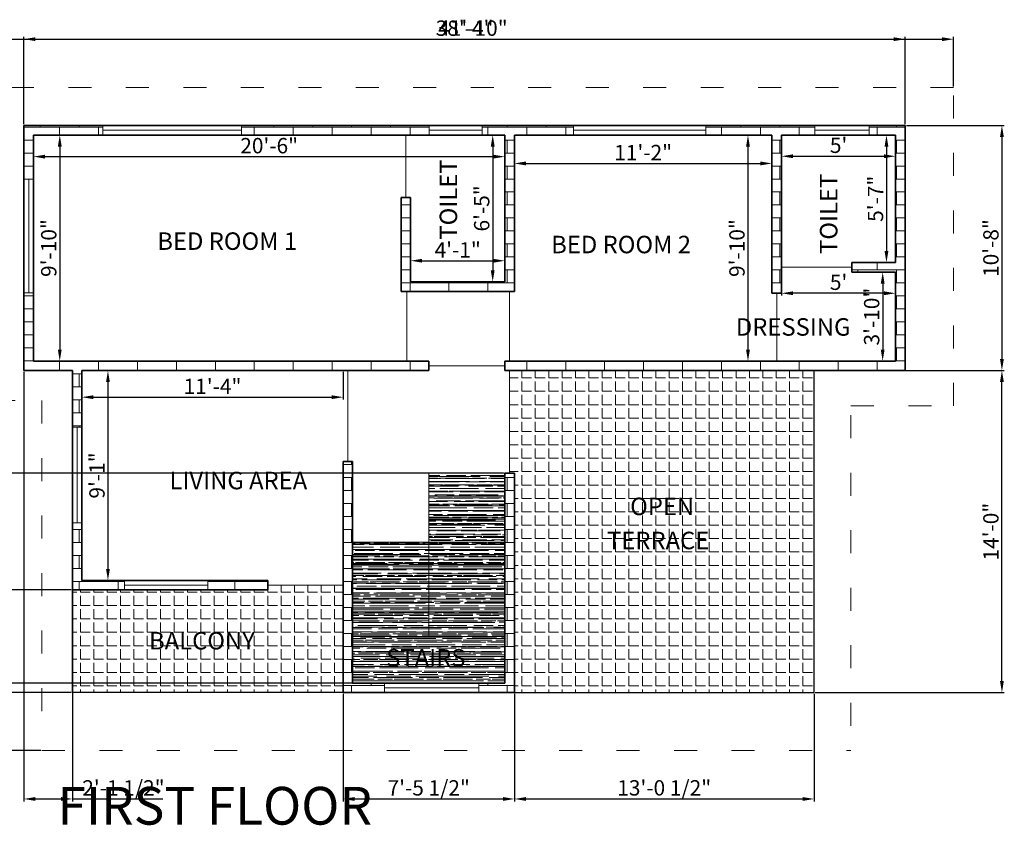
# Model space of a CAD drawing. Units: millimetres. Extents: x 1518 to 2850, y 936 to 2174.
# Tile 5 of 5: x 2336 to 2850, y 1715 to 2136. Entities that reach past the tile are written whole.
import ezdxf

# ---------------------------------------------------------------- set-up
doc = ezdxf.new("R2010")
doc.units = ezdxf.units.MM
doc.linetypes.add('ACAD_ISO03W100', pattern=[30, 12, -18])
for name, color, linetype, lineweight, true_color in [('A-ANNO-DIMS', 9, 'Continuous', 18, 0xafd9aa), ('A-ANNO-TEXT', 85, 'Continuous', 25, 0x58ba48), ('A-AREA-IDEN', 31, 'Continuous', 18, 0xfecc66), ('A-DOOR', 244, 'Continuous', 20, 0x991b1e), ('A-FLOR-PATT', 252, 'Continuous', 13, 0x939598), ('A-GLAZ', 141, 'Continuous', 18, 0xadddf7), ('A-ROOF-OVHD', 177, 'ACAD_ISO03W100', 18, 0x293189)]:
    doc.layers.add(name, color=color, linetype=linetype, lineweight=lineweight, true_color=true_color)
for name, color, linetype, lineweight in [('A-FLOR', 7, 'Continuous', 25), ('A-FLOR-STRS', 7, 'Continuous', 20), ('A-FLOR-STRS-PATT', 7, 'Continuous', 13), ('A-WALL', 7, 'Continuous', 35), ('A-WALL-PATT', 7, 'Continuous', 13)]:
    doc.layers.add(name, color=color, linetype=linetype, lineweight=lineweight)
doc.styles.get("Standard").update_dxf_attribs({"font": 'arial.ttf'})
doc.dimstyles.new('ISO-25', dxfattribs={"dimtxt": 8, "dimasz": 6, "dimexe": 1.25, "dimexo": 0.625, "dimtad": 1, "dimdec": 0, "dimlunit": 3, "dimtxsty": 'Standard', "dimcen": 2.5, "dimadec": 0, "dimazin": 0, "dimtfac": 1, "dimtdec": 0, "dimtmove": 0, "dimatfit": 3, "dimfxl": 1, "dimarcsym": 0})

# ---------------------------------------------------------------- blocks, each defined once
blk = doc.blocks.new('*D14')
at = {"layer": 'A-ANNO-DIMS', "color": 0, "lineweight": -2, "transparency": 16777216}
for p, q in [((2343.49, 2074.9), (2343.49, 2062.99)), ((2589.49, 2074.9), (2589.49, 2062.99)), ((2349.49, 2064.24), (2583.49, 2064.24))]:
    blk.add_line(p, q, dxfattribs=at)
at = {"layer": 'A-ANNO-DIMS', "color": 0, "transparency": 16777216}
for points in [[(2349.49, 2065.24), (2349.49, 2063.24), (2343.49, 2064.24)], [(2583.49, 2065.24), (2583.49, 2063.24), (2589.49, 2064.24)]]:
    blk.add_solid(points, dxfattribs=at)
at = {"layer": 'Defpoints', "color": 0, "transparency": 16777216}
for p in [(2343.49, 2075.52), (2589.49, 2075.52), (2589.49, 2064.24)]:
    blk.add_point(p, dxfattribs=at)
at = {"layer": 'A-ANNO-DIMS', "color": 0, "transparency": 16777216, "insert": (2466.49, 2068.95), "char_height": 8, "attachment_point": 5}
blk.add_mtext('20\'-6"', dxfattribs=at)
blk = doc.blocks.new('*D15')
at = {"layer": 'A-ANNO-DIMS', "color": 0, "lineweight": -2, "transparency": 16777216}
for p, q in [((2344.11, 2075.52), (2358.43, 2075.52)), ((2357.18, 2069.52), (2357.18, 1963.6)), ((2344.11, 1957.6), (2358.43, 1957.6))]:
    blk.add_line(p, q, dxfattribs=at)
at = {"layer": 'A-ANNO-DIMS', "color": 0, "transparency": 16777216}
for points in [[(2356.18, 2069.52), (2358.18, 2069.52), (2357.18, 2075.52)], [(2356.18, 1963.6), (2358.18, 1963.6), (2357.18, 1957.6)]]:
    blk.add_solid(points, dxfattribs=at)
at = {"layer": 'Defpoints', "color": 0, "transparency": 16777216}
for p in [(2343.49, 2075.52), (2343.49, 1957.6), (2357.18, 1957.6)]:
    blk.add_point(p, dxfattribs=at)
at = {"layer": 'A-ANNO-DIMS', "color": 0, "transparency": 16777216, "insert": (2352.47, 2016.56), "char_height": 8, "attachment_point": 5, "rotation": 90}
blk.add_mtext('9\'-10"', dxfattribs=at)
blk = doc.blocks.new('*D16')
at = {"layer": 'A-ANNO-DIMS', "color": 0, "lineweight": -2, "transparency": 16777216}
for p, q in [((2588.86, 2075.52), (2581.93, 2075.52)), ((2583.18, 2069.52), (2583.18, 2004.95)), ((2588.86, 1998.95), (2581.93, 1998.95))]:
    blk.add_line(p, q, dxfattribs=at)
at = {"layer": 'A-ANNO-DIMS', "color": 0, "transparency": 16777216}
for points in [[(2582.18, 2069.52), (2584.18, 2069.52), (2583.18, 2075.52)], [(2582.18, 2004.95), (2584.18, 2004.95), (2583.18, 1998.95)]]:
    blk.add_solid(points, dxfattribs=at)
at = {"layer": 'Defpoints', "color": 0, "transparency": 16777216}
for p in [(2589.49, 2075.52), (2583.18, 1998.95), (2589.49, 1998.95)]:
    blk.add_point(p, dxfattribs=at)
at = {"layer": 'A-ANNO-DIMS', "color": 0, "transparency": 16777216, "insert": (2578.47, 2037.24), "char_height": 8, "attachment_point": 5, "rotation": 90}
blk.add_mtext('6\'-5"', dxfattribs=at)
blk = doc.blocks.new('*D17')
at = {"layer": 'A-ANNO-DIMS', "color": 0, "lineweight": -2, "transparency": 16777216}
for p, q in [((2540.33, 1999.58), (2540.33, 2011.19)), ((2546.33, 2009.94), (2583.49, 2009.94)), ((2589.49, 1999.58), (2589.49, 2011.19))]:
    blk.add_line(p, q, dxfattribs=at)
at = {"layer": 'A-ANNO-DIMS', "color": 0, "transparency": 16777216}
for points in [[(2546.33, 2010.94), (2546.33, 2008.94), (2540.33, 2009.94)], [(2583.49, 2010.94), (2583.49, 2008.94), (2589.49, 2009.94)]]:
    blk.add_solid(points, dxfattribs=at)
at = {"layer": 'Defpoints', "color": 0, "transparency": 16777216}
for p in [(2589.49, 2009.94), (2540.33, 1998.95), (2589.49, 1998.95)]:
    blk.add_point(p, dxfattribs=at)
at = {"layer": 'A-ANNO-DIMS', "color": 0, "transparency": 16777216, "insert": (2564.91, 2014.59), "char_height": 8, "attachment_point": 5}
blk.add_mtext('4\'-1"', dxfattribs=at)
blk = doc.blocks.new('*D18')
at = {"layer": 'A-ANNO-DIMS', "color": 0, "lineweight": -2, "transparency": 16777216}
for p, q in [((2594.49, 2074.9), (2594.49, 2059.46)), ((2728.96, 2074.9), (2728.96, 2059.46)), ((2600.49, 2060.71), (2722.96, 2060.71))]:
    blk.add_line(p, q, dxfattribs=at)
at = {"layer": 'A-ANNO-DIMS', "color": 0, "transparency": 16777216}
for points in [[(2600.49, 2061.71), (2600.49, 2059.71), (2594.49, 2060.71)], [(2722.96, 2061.71), (2722.96, 2059.71), (2728.96, 2060.71)]]:
    blk.add_solid(points, dxfattribs=at)
at = {"layer": 'Defpoints', "color": 0, "transparency": 16777216}
for p in [(2594.49, 2075.52), (2728.96, 2075.52), (2728.96, 2060.71)]:
    blk.add_point(p, dxfattribs=at)
at = {"layer": 'A-ANNO-DIMS', "color": 0, "transparency": 16777216, "insert": (2661.72, 2065.35), "char_height": 8, "attachment_point": 5}
blk.add_mtext('11\'-2"', dxfattribs=at)
blk = doc.blocks.new('*D19')
at = {"layer": 'A-ANNO-DIMS', "color": 0, "lineweight": -2, "transparency": 16777216}
for p, q in [((2728.33, 2075.52), (2715.17, 2075.52)), ((2716.42, 2069.52), (2716.42, 1963.6)), ((2728.33, 1957.6), (2715.17, 1957.6))]:
    blk.add_line(p, q, dxfattribs=at)
at = {"layer": 'A-ANNO-DIMS', "color": 0, "transparency": 16777216}
for points in [[(2715.42, 2069.52), (2717.42, 2069.52), (2716.42, 2075.52)], [(2715.42, 1963.6), (2717.42, 1963.6), (2716.42, 1957.6)]]:
    blk.add_solid(points, dxfattribs=at)
at = {"layer": 'Defpoints', "color": 0, "transparency": 16777216}
for p in [(2728.96, 2075.52), (2716.42, 1957.6), (2728.96, 1957.6)]:
    blk.add_point(p, dxfattribs=at)
at = {"layer": 'A-ANNO-DIMS', "color": 0, "transparency": 16777216, "insert": (2711.71, 2016.56), "char_height": 8, "attachment_point": 5, "rotation": 90}
blk.add_mtext('9\'-10"', dxfattribs=at)
blk = doc.blocks.new('*D20')
at = {"layer": 'A-ANNO-DIMS', "color": 0, "lineweight": -2, "transparency": 16777216}
for p, q in [((2733.96, 2074.9), (2733.96, 2063.2)), ((2793.49, 2074.9), (2793.49, 2063.2)), ((2739.96, 2064.45), (2787.49, 2064.45))]:
    blk.add_line(p, q, dxfattribs=at)
at = {"layer": 'A-ANNO-DIMS', "color": 0, "transparency": 16777216}
for points in [[(2739.96, 2065.45), (2739.96, 2063.45), (2733.96, 2064.45)], [(2787.49, 2065.45), (2787.49, 2063.45), (2793.49, 2064.45)]]:
    blk.add_solid(points, dxfattribs=at)
at = {"layer": 'Defpoints', "color": 0, "transparency": 16777216}
for p in [(2733.96, 2075.52), (2793.49, 2075.52), (2793.49, 2064.45)]:
    blk.add_point(p, dxfattribs=at)
at = {"layer": 'A-ANNO-DIMS', "color": 0, "transparency": 16777216, "insert": (2763.72, 2069.15), "char_height": 8, "attachment_point": 5}
blk.add_mtext("5'", dxfattribs=at)
blk = doc.blocks.new('*D21')
at = {"layer": 'A-ANNO-DIMS', "color": 0, "lineweight": -2, "transparency": 16777216}
for p, q in [((2792.86, 2075.52), (2787.47, 2075.52)), ((2788.72, 2069.52), (2788.72, 2015.01)), ((2792.86, 2009.01), (2787.47, 2009.01))]:
    blk.add_line(p, q, dxfattribs=at)
at = {"layer": 'A-ANNO-DIMS', "color": 0, "transparency": 16777216}
for points in [[(2787.72, 2069.52), (2789.72, 2069.52), (2788.72, 2075.52)], [(2787.72, 2015.01), (2789.72, 2015.01), (2788.72, 2009.01)]]:
    blk.add_solid(points, dxfattribs=at)
at = {"layer": 'Defpoints', "color": 0, "transparency": 16777216}
for p in [(2793.49, 2075.52), (2788.72, 2009.01), (2793.49, 2009.01)]:
    blk.add_point(p, dxfattribs=at)
at = {"layer": 'A-ANNO-DIMS', "color": 0, "transparency": 16777216, "insert": (2784.03, 2042.27), "char_height": 8, "attachment_point": 5, "rotation": 90}
blk.add_mtext('5\'-7"', dxfattribs=at)
blk = doc.blocks.new('*D22')
at = {"layer": 'A-ANNO-DIMS', "color": 0, "lineweight": -2, "transparency": 16777216}
for p, q in [((2733.96, 2003.39), (2733.96, 1991.73)), ((2793.49, 2003.39), (2793.49, 1991.73)), ((2787.49, 1992.98), (2739.96, 1992.98))]:
    blk.add_line(p, q, dxfattribs=at)
at = {"layer": 'A-ANNO-DIMS', "color": 0, "transparency": 16777216}
for points in [[(2739.96, 1993.98), (2739.96, 1991.98), (2733.96, 1992.98)], [(2787.49, 1993.98), (2787.49, 1991.98), (2793.49, 1992.98)]]:
    blk.add_solid(points, dxfattribs=at)
at = {"layer": 'Defpoints', "color": 0, "transparency": 16777216}
for p in [(2733.96, 2004.01), (2793.49, 2004.01), (2733.96, 1992.98)]:
    blk.add_point(p, dxfattribs=at)
at = {"layer": 'A-ANNO-DIMS', "color": 0, "transparency": 16777216, "insert": (2763.72, 1997.67), "char_height": 8, "attachment_point": 5}
blk.add_mtext("5'", dxfattribs=at)
blk = doc.blocks.new('*D23')
at = {"layer": 'A-ANNO-DIMS', "color": 0, "lineweight": -2, "transparency": 16777216}
for p, q in [((2792.86, 2004.01), (2785.49, 2004.01)), ((2786.74, 1998.01), (2786.74, 1963.6)), ((2792.86, 1957.6), (2785.49, 1957.6))]:
    blk.add_line(p, q, dxfattribs=at)
at = {"layer": 'A-ANNO-DIMS', "color": 0, "transparency": 16777216}
for points in [[(2785.74, 1998.01), (2787.74, 1998.01), (2786.74, 2004.01)], [(2785.74, 1963.6), (2787.74, 1963.6), (2786.74, 1957.6)]]:
    blk.add_solid(points, dxfattribs=at)
at = {"layer": 'Defpoints', "color": 0, "transparency": 16777216}
for p in [(2793.49, 2004.01), (2786.74, 1957.6), (2793.49, 1957.6)]:
    blk.add_point(p, dxfattribs=at)
at = {"layer": 'A-ANNO-DIMS', "color": 0, "transparency": 16777216, "insert": (2782.03, 1980.8), "char_height": 8, "attachment_point": 5, "rotation": 90}
blk.add_mtext('3\'-10"', dxfattribs=at)
blk = doc.blocks.new('*D24')
at = {"layer": 'A-ANNO-DIMS', "color": 0, "lineweight": -2, "transparency": 16777216}
for p, q in [((2369.38, 1952.6), (2383.59, 1952.6)), ((2382.34, 1946.6), (2382.34, 1849.2)), ((2369.38, 1843.2), (2383.59, 1843.2))]:
    blk.add_line(p, q, dxfattribs=at)
at = {"layer": 'A-ANNO-DIMS', "color": 0, "transparency": 16777216}
for points in [[(2381.34, 1946.6), (2383.34, 1946.6), (2382.34, 1952.6)], [(2381.34, 1849.2), (2383.34, 1849.2), (2382.34, 1843.2)]]:
    blk.add_solid(points, dxfattribs=at)
at = {"layer": 'Defpoints', "color": 0, "transparency": 16777216}
for p in [(2368.76, 1952.6), (2368.76, 1843.2), (2382.34, 1843.2)]:
    blk.add_point(p, dxfattribs=at)
at = {"layer": 'A-ANNO-DIMS', "color": 0, "transparency": 16777216, "insert": (2377.63, 1897.9), "char_height": 8, "attachment_point": 5, "rotation": 90}
blk.add_mtext('9\'-1"', dxfattribs=at)
blk = doc.blocks.new('*D25')
at = {"layer": 'A-ANNO-DIMS', "color": 0, "lineweight": -2, "transparency": 16777216}
for p, q in [((2368.76, 1951.97), (2368.76, 1937.5)), ((2505.07, 1951.97), (2505.07, 1937.5)), ((2374.76, 1938.75), (2499.07, 1938.75))]:
    blk.add_line(p, q, dxfattribs=at)
at = {"layer": 'A-ANNO-DIMS', "color": 0, "transparency": 16777216}
for points in [[(2374.76, 1939.75), (2374.76, 1937.75), (2368.76, 1938.75)], [(2499.07, 1939.75), (2499.07, 1937.75), (2505.07, 1938.75)]]:
    blk.add_solid(points, dxfattribs=at)
at = {"layer": 'Defpoints', "color": 0, "transparency": 16777216}
for p in [(2368.76, 1952.6), (2505.07, 1952.6), (2505.07, 1938.75)]:
    blk.add_point(p, dxfattribs=at)
at = {"layer": 'A-ANNO-DIMS', "color": 0, "transparency": 16777216, "insert": (2436.92, 1943.39), "char_height": 8, "attachment_point": 5}
blk.add_mtext('11\'-4"', dxfattribs=at)
blk = doc.blocks.new('*D42')
at = {"layer": 'A-ANNO-DIMS', "color": 0, "lineweight": -2, "transparency": 16777216}
for p, q in [((2338.49, 2081.15), (2338.49, 2126.78)), ((2344.49, 2125.53), (2792.49, 2125.53)), ((2798.49, 2081.15), (2798.49, 2126.78))]:
    blk.add_line(p, q, dxfattribs=at)
at = {"layer": 'A-ANNO-DIMS', "color": 0, "transparency": 16777216}
for points in [[(2344.49, 2126.53), (2344.49, 2124.53), (2338.49, 2125.53)], [(2792.49, 2126.53), (2792.49, 2124.53), (2798.49, 2125.53)]]:
    blk.add_solid(points, dxfattribs=at)
at = {"layer": 'Defpoints', "color": 0, "transparency": 16777216}
for p in [(2798.49, 2125.53), (2338.49, 2080.52), (2798.49, 2080.52)]:
    blk.add_point(p, dxfattribs=at)
at = {"layer": 'A-ANNO-DIMS', "color": 0, "transparency": 16777216, "insert": (2568.49, 2130.24), "char_height": 8, "attachment_point": 5}
blk.add_mtext('38\'-4"', dxfattribs=at)
blk = doc.blocks.new('*D43')
at = {"layer": 'A-ANNO-DIMS', "color": 0, "lineweight": -2, "transparency": 16777216}
for p, q in [((2799.11, 2080.52), (2850.23, 2080.52)), ((2848.98, 2074.52), (2848.98, 1958.6)), ((2799.11, 1952.6), (2850.23, 1952.6))]:
    blk.add_line(p, q, dxfattribs=at)
at = {"layer": 'A-ANNO-DIMS', "color": 0, "transparency": 16777216}
for points in [[(2847.98, 2074.52), (2849.98, 2074.52), (2848.98, 2080.52)], [(2847.98, 1958.6), (2849.98, 1958.6), (2848.98, 1952.6)]]:
    blk.add_solid(points, dxfattribs=at)
at = {"layer": 'Defpoints', "color": 0, "transparency": 16777216}
for p in [(2798.49, 2080.52), (2798.49, 1952.6), (2848.98, 1952.6)]:
    blk.add_point(p, dxfattribs=at)
at = {"layer": 'A-ANNO-DIMS', "color": 0, "transparency": 16777216, "insert": (2844.27, 2016.56), "char_height": 8, "attachment_point": 5, "rotation": 90}
blk.add_mtext('10\'-8"', dxfattribs=at)
blk = doc.blocks.new('*D44')
at = {"layer": 'A-ANNO-DIMS', "color": 0, "lineweight": -2, "transparency": 16777216}
for p, q in [((2338.49, 1951.97), (2338.49, 1727.89)), ((2363.76, 1951.97), (2363.76, 1727.89)), ((2344.49, 1729.14), (2357.76, 1729.14)), ((2363.76, 1729.14), (2411.05, 1729.14))]:
    blk.add_line(p, q, dxfattribs=at)
at = {"layer": 'A-ANNO-DIMS', "color": 0, "transparency": 16777216}
for points in [[(2344.49, 1730.14), (2344.49, 1728.14), (2338.49, 1729.14)], [(2357.76, 1730.14), (2357.76, 1728.14), (2363.76, 1729.14)]]:
    blk.add_solid(points, dxfattribs=at)
at = {"layer": 'Defpoints', "color": 0, "transparency": 16777216}
for p in [(2338.49, 1952.6), (2363.76, 1952.6), (2363.76, 1729.14)]:
    blk.add_point(p, dxfattribs=at)
at = {"layer": 'A-ANNO-DIMS', "color": 0, "transparency": 16777216, "insert": (2390.41, 1733.9), "char_height": 8, "attachment_point": 5}
blk.add_mtext('2\'-1 1/2"', dxfattribs=at)
blk = doc.blocks.new('*D45')
at = {"layer": 'A-ANNO-DIMS', "color": 0, "lineweight": -2, "transparency": 16777216}
for p, q in [((2505.07, 1783.97), (2505.07, 1727.89)), ((2594.49, 1783.97), (2594.49, 1727.89)), ((2511.07, 1729.14), (2588.49, 1729.14))]:
    blk.add_line(p, q, dxfattribs=at)
at = {"layer": 'A-ANNO-DIMS', "color": 0, "transparency": 16777216}
for points in [[(2511.07, 1730.14), (2511.07, 1728.14), (2505.07, 1729.14)], [(2588.49, 1730.14), (2588.49, 1728.14), (2594.49, 1729.14)]]:
    blk.add_solid(points, dxfattribs=at)
at = {"layer": 'Defpoints', "color": 0, "transparency": 16777216}
for p in [(2505.07, 1784.6), (2594.49, 1784.6), (2594.49, 1729.14)]:
    blk.add_point(p, dxfattribs=at)
at = {"layer": 'A-ANNO-DIMS', "color": 0, "transparency": 16777216, "insert": (2549.78, 1733.9), "char_height": 8, "attachment_point": 5}
blk.add_mtext('7\'-5 1/2"', dxfattribs=at)
blk = doc.blocks.new('*D46')
at = {"layer": 'A-ANNO-DIMS', "color": 0, "lineweight": -2, "transparency": 16777216}
for p, q in [((2594.49, 1783.97), (2594.49, 1727.89)), ((2750.92, 1783.97), (2750.92, 1727.89)), ((2600.49, 1729.14), (2744.92, 1729.14))]:
    blk.add_line(p, q, dxfattribs=at)
at = {"layer": 'A-ANNO-DIMS', "color": 0, "transparency": 16777216}
for points in [[(2600.49, 1730.14), (2600.49, 1728.14), (2594.49, 1729.14)], [(2744.92, 1730.14), (2744.92, 1728.14), (2750.92, 1729.14)]]:
    blk.add_solid(points, dxfattribs=at)
at = {"layer": 'Defpoints', "color": 0, "transparency": 16777216}
for p in [(2594.49, 1784.6), (2750.92, 1784.6), (2750.92, 1729.14)]:
    blk.add_point(p, dxfattribs=at)
at = {"layer": 'A-ANNO-DIMS', "color": 0, "transparency": 16777216, "insert": (2672.7, 1733.91), "char_height": 8, "attachment_point": 5}
blk.add_mtext('13\'-0 1/2"', dxfattribs=at)
blk = doc.blocks.new('*D47')
at = {"layer": 'A-ANNO-DIMS', "color": 0, "lineweight": -2, "transparency": 16777216}
for p, q in [((2751.54, 1952.6), (2850.23, 1952.6)), ((2848.98, 1790.6), (2848.98, 1946.6)), ((2751.54, 1784.6), (2850.23, 1784.6))]:
    blk.add_line(p, q, dxfattribs=at)
at = {"layer": 'A-ANNO-DIMS', "color": 0, "transparency": 16777216}
for points in [[(2847.98, 1946.6), (2849.98, 1946.6), (2848.98, 1952.6)], [(2847.98, 1790.6), (2849.98, 1790.6), (2848.98, 1784.6)]]:
    blk.add_solid(points, dxfattribs=at)
at = {"layer": 'Defpoints', "color": 0, "transparency": 16777216}
for p in [(2750.92, 1952.6), (2848.98, 1952.6), (2750.92, 1784.6)]:
    blk.add_point(p, dxfattribs=at)
at = {"layer": 'A-ANNO-DIMS', "color": 0, "transparency": 16777216, "insert": (2844.27, 1868.6), "char_height": 8, "attachment_point": 5, "rotation": 90}
blk.add_mtext('14\'-0"', dxfattribs=at)
blk = doc.blocks.new('*D48')
at = {"layer": 'A-ANNO-DIMS', "color": 0, "lineweight": -2, "transparency": 16777216}
for p, q in [((2588.86, 1899.05), (2295.47, 1899.05)), ((2296.72, 1795.6), (2296.72, 1893.05)), ((2588.86, 1789.6), (2295.47, 1789.6))]:
    blk.add_line(p, q, dxfattribs=at)
at = {"layer": 'A-ANNO-DIMS', "color": 0, "transparency": 16777216}
for points in [[(2295.72, 1893.05), (2297.72, 1893.05), (2296.72, 1899.05)], [(2295.72, 1795.6), (2297.72, 1795.6), (2296.72, 1789.6)]]:
    blk.add_solid(points, dxfattribs=at)
at = {"layer": 'Defpoints', "color": 0, "transparency": 16777216}
for p in [(2296.72, 1899.05), (2589.49, 1899.05), (2589.49, 1789.6)]:
    blk.add_point(p, dxfattribs=at)
at = {"layer": 'A-ANNO-DIMS', "color": 0, "transparency": 16777216, "insert": (2291.96, 1844.32), "char_height": 8, "attachment_point": 5, "rotation": 90}
blk.add_mtext('9\'-1 1/2"', dxfattribs=at)
blk = doc.blocks.new('*D49')
at = {"layer": 'A-ANNO-DIMS', "color": 0, "lineweight": -2, "transparency": 16777216}
for p, q in [((2363.13, 1838.2), (2295.47, 1838.2)), ((2296.72, 1790.6), (2296.72, 1832.2)), ((2363.13, 1784.6), (2295.47, 1784.6))]:
    blk.add_line(p, q, dxfattribs=at)
at = {"layer": 'A-ANNO-DIMS', "color": 0, "transparency": 16777216}
for points in [[(2295.72, 1832.2), (2297.72, 1832.2), (2296.72, 1838.2)], [(2295.72, 1790.6), (2297.72, 1790.6), (2296.72, 1784.6)]]:
    blk.add_solid(points, dxfattribs=at)
at = {"layer": 'Defpoints', "color": 0, "transparency": 16777216}
for p in [(2296.72, 1838.2), (2363.76, 1838.2), (2363.76, 1784.6)]:
    blk.add_point(p, dxfattribs=at)
at = {"layer": 'A-ANNO-DIMS', "color": 0, "transparency": 16777216, "insert": (2291.96, 1811.4), "char_height": 8, "attachment_point": 5, "rotation": 90}
blk.add_mtext('4\'-5 1/2"', dxfattribs=at)
blk = doc.blocks.new('*D50')
at = {"layer": 'A-ANNO-DIMS', "color": 0, "lineweight": -2, "transparency": 16777216}
for p, q in [((2321.97, 2100.9), (2321.97, 2126.78)), ((2327.97, 2125.53), (2817.73, 2125.53)), ((2823.73, 2100.9), (2823.73, 2126.78))]:
    blk.add_line(p, q, dxfattribs=at)
at = {"layer": 'A-ANNO-DIMS', "color": 0, "transparency": 16777216}
for points in [[(2327.97, 2126.53), (2327.97, 2124.53), (2321.97, 2125.53)], [(2817.73, 2126.53), (2817.73, 2124.53), (2823.73, 2125.53)]]:
    blk.add_solid(points, dxfattribs=at)
at = {"layer": 'Defpoints', "color": 0, "transparency": 16777216}
for p in [(2823.73, 2125.53), (2321.97, 2100.28), (2823.73, 2100.28)]:
    blk.add_point(p, dxfattribs=at)
at = {"layer": 'A-ANNO-DIMS', "color": 0, "transparency": 16777216, "insert": (2572.85, 2130.24), "char_height": 8, "attachment_point": 5}
blk.add_mtext('41\'-10"', dxfattribs=at)
blk = doc.blocks.new('*D51')
at = {"layer": 'A-ANNO-DIMS', "color": 0, "lineweight": -2, "transparency": 16777216}
for p, q in [((2321.34, 2100.28), (2295.47, 2100.28)), ((2296.72, 2094.28), (2296.72, 1760.39)), ((2347.23, 1754.39), (2295.47, 1754.39))]:
    blk.add_line(p, q, dxfattribs=at)
at = {"layer": 'A-ANNO-DIMS', "color": 0, "transparency": 16777216}
for points in [[(2295.72, 2094.28), (2297.72, 2094.28), (2296.72, 2100.28)], [(2295.72, 1760.39), (2297.72, 1760.39), (2296.72, 1754.39)]]:
    blk.add_solid(points, dxfattribs=at)
at = {"layer": 'Defpoints', "color": 0, "transparency": 16777216}
for p in [(2321.97, 2100.28), (2296.72, 1754.39), (2347.86, 1754.39)]:
    blk.add_point(p, dxfattribs=at)
at = {"layer": 'A-ANNO-DIMS', "color": 0, "transparency": 16777216, "insert": (2292.01, 1927.34), "char_height": 8, "attachment_point": 5, "rotation": 90}
blk.add_mtext('28\'-10"', dxfattribs=at)

msp = doc.modelspace()

# ---------------------------------------------------------------- hatches: boundary and pattern name
at = {"layer": 'A-FLOR-PATT'}
h = msp.add_hatch(dxfattribs=at)
h.set_pattern_fill('ANGLE', color=256)
h.set_pattern_definition([(0, (0, 0), (0, 6.985), [5.08, -1.905]), (90, (0, 0), (-6.985, 4e-16), [5.08, -1.905])])
h.paths.add_polyline_path([(2505.07, 1838.2), (2505.07, 1840.7), (2465.77, 1840.7), (2465.77, 1838.2), (2363.76, 1838.2), (2363.76, 1784.6), (2505.07, 1784.6)])
h.paths.add_polyline_path([(2750.92, 1952.6), (2594.49, 1952.6), (2591.99, 1952.6), (2591.99, 1899.05), (2594.49, 1899.05), (2594.49, 1784.6), (2750.92, 1784.6)])
at = {"layer": 'A-FLOR-STRS-PATT'}
h = msp.add_hatch(dxfattribs=at)
h.set_pattern_fill('AR-RROOF', color=256, scale=0.1)
h.paths.add_polyline_path([(2549.78, 1863.05), (2510.07, 1863.05), (2510.07, 1851.05), (2549.78, 1851.05)])
h.paths.add_polyline_path([(2589.49, 1899.05), (2549.78, 1899.05), (2549.78, 1887.05), (2589.49, 1887.05)])
h.paths.add_polyline_path([(2589.49, 1887.05), (2549.78, 1887.05), (2549.78, 1875.05), (2589.49, 1875.05)])
h.paths.add_polyline_path([(2589.49, 1875.05), (2549.78, 1875.05), (2549.78, 1863.05), (2589.49, 1863.05)])
h.paths.add_polyline_path([(2589.49, 1863.05), (2549.78, 1863.05), (2549.78, 1851.05), (2589.49, 1851.05)])
h.paths.add_polyline_path([(2589.49, 1851.05), (2549.78, 1851.05), (2549.78, 1839.05), (2589.49, 1839.05)])
h.paths.add_polyline_path([(2589.49, 1839.05), (2549.78, 1839.05), (2549.78, 1827.05), (2589.49, 1827.05)])
h.paths.add_polyline_path([(2589.49, 1827.05), (2549.78, 1827.05), (2549.78, 1813.9), (2589.49, 1813.9)])
h.paths.add_polyline_path([(2589.49, 1813.9), (2549.78, 1813.9), (2510.07, 1813.9), (2510.07, 1789.6), (2589.49, 1789.6)])
h.paths.add_polyline_path([(2549.78, 1827.05), (2510.07, 1827.05), (2510.07, 1813.9), (2549.78, 1813.9)])
h.paths.add_polyline_path([(2549.78, 1839.05), (2510.07, 1839.05), (2510.07, 1827.05), (2549.78, 1827.05)])
h.paths.add_polyline_path([(2549.78, 1851.05), (2510.07, 1851.05), (2510.07, 1839.05), (2549.78, 1839.05)])
at = {"layer": 'A-WALL-PATT'}
h = msp.add_hatch(dxfattribs=at)
h.set_pattern_fill('AR-BRSTD', color=256, scale=0.1)
h.paths.add_polyline_path([(2550.01, 2080.52), (2452.04, 2080.52), (2452.04, 2075.52), (2535.33, 2075.52), (2540.33, 2075.52), (2550.01, 2075.52)])
h.paths.add_polyline_path([(2379.7, 2080.52), (2338.49, 2080.52), (2338.49, 2052.54), (2343.49, 2052.54), (2343.49, 2075.52), (2379.7, 2075.52)])
h.paths.add_polyline_path([(2549.78, 1957.6), (2343.49, 1957.6), (2343.49, 1993.2), (2338.49, 1993.2), (2338.49, 1952.6), (2363.76, 1952.6), (2363.76, 1923.14), (2368.76, 1923.14), (2368.76, 1952.6), (2505.07, 1952.6), (2510.07, 1952.6), (2549.78, 1952.6)])
h.paths.add_polyline_path([(2625.42, 2080.52), (2594.49, 2080.52), (2577.67, 2080.52), (2577.67, 2075.52), (2589.49, 2075.52), (2589.49, 1998.95), (2540.33, 1998.95), (2540.33, 2043), (2535.33, 2043), (2535.33, 1993.95), (2589.49, 1993.95), (2594.49, 1993.92), (2594.49, 2075.52), (2625.42, 2075.52)])
h.paths.add_polyline_path([(2751.28, 2080.52), (2694.39, 2080.52), (2694.39, 2075.52), (2728.96, 2075.52), (2728.96, 1992.98), (2733.96, 1992.98), (2733.96, 2004.01), (2733.96, 2009.01), (2733.96, 2075.52), (2751.28, 2075.52)], flags=17)
h.paths.add_polyline_path([(2798.49, 2080.52), (2779.63, 2080.52), (2779.63, 2075.52), (2793.49, 2075.52), (2793.49, 2009.01), (2770.7, 2009.01), (2770.7, 2004.01), (2793.49, 2004.01), (2793.49, 1957.6), (2733.96, 1957.6), (2728.96, 1957.6), (2594.49, 1957.6), (2589.49, 1957.6), (2589.49, 1952.6), (2594.49, 1952.6), (2798.49, 1952.6)])
h.paths.add_polyline_path([(2368.76, 1873.29), (2363.76, 1873.29), (2363.76, 1838.2), (2391.06, 1838.2), (2391.06, 1843.2), (2368.76, 1843.2)])
h.paths.add_polyline_path([(2465.77, 1843.2), (2434.42, 1843.2), (2434.42, 1838.2), (2465.77, 1838.2)])
h.paths.add_polyline_path([(2510.07, 1905.25), (2505.07, 1905.25), (2505.07, 1843.2), (2505.07, 1838.2), (2505.07, 1784.6), (2526.69, 1784.6), (2526.69, 1789.6), (2510.07, 1789.6), (2510.07, 1838.2), (2510.07, 1839.05)])
h.paths.add_polyline_path([(2594.49, 1899.05), (2589.49, 1899.05), (2589.49, 1887.05), (2589.49, 1789.6), (2575.94, 1789.6), (2575.94, 1784.6), (2594.49, 1784.6)])

# ---------------------------------------------------------------- linework, layer by layer
at = {"layer": 'A-DOOR'}
for p, q in [((2537.83, 2043), (2537.83, 2075.52)), ((2770.7, 2006.51), (2733.96, 2006.51)), ((2538.39, 1993.95), (2538.39, 1957.6)), ((2591.99, 1957.6), (2591.99, 1993.92)), ((2731.46, 1992.98), (2731.46, 1957.6)), ((2549.78, 1955.1), (2589.49, 1955.1)), ((2507.57, 1905.25), (2507.57, 1952.6)), ((2591.99, 1899.05), (2591.99, 1952.6)), ((2465.77, 1840.7), (2505.07, 1840.7))]:
    msp.add_line(p, q, dxfattribs=at)
at = {"layer": 'A-FLOR'}
for p, q in [((2750.92, 1784.6), (2750.92, 1952.6)), ((2363.76, 1784.6), (2363.76, 1838.2)), ((2505.07, 1784.6), (2363.76, 1784.6)), ((2594.49, 1784.6), (2750.92, 1784.6))]:
    msp.add_line(p, q, dxfattribs=at)
at = {"layer": 'A-FLOR-STRS'}
for p, q in [((2549.78, 1813.9), (2549.78, 1899.05)), ((2549.78, 1899.05), (2589.49, 1899.05)), ((2589.49, 1899.05), (2589.49, 1887.05)), ((2589.49, 1887.05), (2549.78, 1887.05)), ((2549.78, 1887.05), (2549.78, 1875.05)), ((2549.78, 1875.05), (2589.49, 1875.05)), ((2589.49, 1875.05), (2589.49, 1863.05)), ((2589.49, 1863.05), (2510.07, 1863.05)), ((2510.07, 1863.05), (2510.07, 1851.05)), ((2510.07, 1851.05), (2589.49, 1851.05)), ((2589.49, 1851.05), (2589.49, 1839.05)), ((2589.49, 1839.05), (2510.07, 1839.05)), ((2510.07, 1839.05), (2510.07, 1827.05)), ((2510.07, 1827.05), (2589.49, 1827.05)), ((2510.07, 1813.9), (2589.49, 1813.9))]:
    msp.add_line(p, q, dxfattribs=at)
at = {"layer": 'A-GLAZ'}
for p, q in [((2379.7, 2078.02), (2452.04, 2078.02)), ((2550.01, 2078.02), (2577.67, 2078.02)), ((2625.42, 2078.02), (2694.39, 2078.02)), ((2751.28, 2078.02), (2779.63, 2078.02)), ((2340.99, 1993.2), (2340.99, 2052.54)), ((2366.26, 1873.29), (2366.26, 1923.14)), ((2391.06, 1840.7), (2434.42, 1840.7)), ((2526.69, 1787.1), (2575.94, 1787.1))]:
    msp.add_line(p, q, dxfattribs=at)
for points in [[(2379.7, 2080.52), (2452.04, 2080.52), (2452.04, 2075.52), (2379.7, 2075.52)], [(2550.01, 2080.52), (2577.67, 2080.52), (2577.67, 2075.52), (2550.01, 2075.52)], [(2625.42, 2080.52), (2694.39, 2080.52), (2694.39, 2075.52), (2625.42, 2075.52)], [(2751.28, 2080.52), (2779.63, 2080.52), (2779.63, 2075.52), (2751.28, 2075.52)], [(2338.49, 2052.54), (2343.49, 2052.54), (2343.49, 1993.2), (2338.49, 1993.2)], [(2363.76, 1923.14), (2368.76, 1923.14), (2368.76, 1873.29), (2363.76, 1873.29)], [(2391.06, 1843.2), (2434.42, 1843.2), (2434.42, 1838.2), (2391.06, 1838.2)], [(2526.69, 1789.6), (2575.94, 1789.6), (2575.94, 1784.6), (2526.69, 1784.6)]]:
    msp.add_lwpolyline(points, close=True, dxfattribs=at)
at = {"layer": 'A-ROOF-OVHD'}
for p, q in [((2823.73, 2100.28), (2321.97, 2100.28)), ((2823.73, 1934.21), (2823.73, 2100.28)), ((2321.97, 1936.95), (2347.86, 1936.95)), ((2347.86, 1936.95), (2347.86, 1767.34)), ((2770.14, 1767.34), (2770.14, 1934.21)), ((2770.14, 1934.21), (2823.73, 1934.21)), ((2347.86, 1754.39), (2770.14, 1754.39))]:
    msp.add_line(p, q, dxfattribs=at)
at = {"layer": 'A-WALL'}
for p, q in [((2338.49, 2080.52), (2338.49, 1952.6)), ((2594.49, 2080.52), (2338.49, 2080.52)), ((2594.49, 2080.52), (2798.49, 2080.52)), ((2798.49, 2080.52), (2798.49, 1952.6)), ((2343.49, 2075.52), (2343.49, 1957.6)), ((2535.33, 2075.52), (2343.49, 2075.52)), ((2589.49, 2075.52), (2540.33, 2075.52)), ((2589.49, 1998.95), (2589.49, 2075.52)), ((2594.49, 1993.92), (2594.49, 2075.52)), ((2594.49, 2075.52), (2728.96, 2075.52)), ((2728.96, 2075.52), (2728.96, 1992.98)), ((2733.96, 2075.52), (2733.96, 2009.01)), ((2733.96, 2075.52), (2793.49, 2075.52)), ((2793.49, 2075.52), (2793.49, 2009.01)), ((2535.33, 2043), (2535.33, 1993.95)), ((2540.33, 2043), (2540.33, 1998.95)), ((2770.7, 2009.01), (2793.49, 2009.01)), ((2733.96, 2004.01), (2733.96, 1992.98)), ((2770.7, 2004.01), (2793.49, 2004.01)), ((2793.49, 2004.01), (2793.49, 1957.6)), ((2540.33, 1998.95), (2589.49, 1998.95)), ((2535.33, 1993.95), (2589.49, 1993.95)), ((2589.49, 1993.92), (2589.49, 1993.95)), ((2343.49, 1957.6), (2549.78, 1957.6)), ((2728.96, 1957.6), (2594.49, 1957.6)), ((2793.49, 1957.6), (2733.96, 1957.6)), ((2338.49, 1952.6), (2363.76, 1952.6)), ((2363.76, 1952.6), (2363.76, 1838.2)), ((2368.76, 1952.6), (2368.76, 1843.2)), ((2368.76, 1952.6), (2505.07, 1952.6)), ((2510.07, 1952.6), (2549.78, 1952.6)), ((2798.49, 1952.6), (2594.49, 1952.6)), ((2505.07, 1843.2), (2505.07, 1905.25)), ((2510.07, 1838.2), (2510.07, 1905.25)), ((2589.49, 1789.6), (2589.49, 1899.05)), ((2594.49, 1784.6), (2594.49, 1899.05)), ((2368.76, 1843.2), (2465.77, 1843.2)), ((2363.76, 1838.2), (2465.77, 1838.2)), ((2505.07, 1838.2), (2505.07, 1784.6)), ((2510.07, 1838.2), (2510.07, 1789.6)), ((2510.07, 1789.6), (2589.49, 1789.6)), ((2505.07, 1784.6), (2594.49, 1784.6))]:
    msp.add_line(p, q, dxfattribs=at)
for points in [[(2535.33, 2075.52), (2540.33, 2075.52)], [(2540.33, 2043), (2535.33, 2043)], [(2733.96, 2004.01), (2733.96, 2004.01), (2733.96, 2009.01)], [(2770.7, 2009.01), (2770.7, 2004.01)], [(2594.49, 1993.92), (2589.49, 1993.92)], [(2733.96, 1992.98), (2728.96, 1992.98)], [(2549.78, 1957.6), (2549.78, 1952.6)], [(2589.49, 1957.6), (2594.49, 1957.6)], [(2589.49, 1952.6), (2589.49, 1957.6)], [(2728.96, 1957.6), (2733.96, 1957.6)], [(2505.07, 1952.6), (2510.07, 1952.6)], [(2589.49, 1952.6), (2594.49, 1952.6)], [(2510.07, 1905.25), (2505.07, 1905.25)], [(2594.49, 1899.05), (2589.49, 1899.05)], [(2465.77, 1843.2), (2465.77, 1838.2)], [(2505.07, 1838.2), (2505.07, 1843.2)]]:
    msp.add_lwpolyline(points, dxfattribs=at)

# ---------------------------------------------------------------- texts
at = {"layer": 'A-ANNO-TEXT'}
msp.add_text('FIRST FLOOR', height=19.6883, dxfattribs=at).set_placement((2356.02, 1715.75))
at = {"layer": 'A-AREA-IDEN'}
for p in [(2564.61, 2020.94), (2763.1, 2013.48)]:
    msp.add_text('TOILET', height=9.117, rotation=90, dxfattribs=at).set_placement(p)
for s, height, p in [('BED ROOM 1', 9.117, (2408.1, 2015.61)), ('BED ROOM 2', 9.117, (2613.7, 2013.84)), ('DRESSING', 9.117, (2710.1, 1970.84)), ('LIVING AREA', 9.1171, (2414.46, 1890.71)), ('OPEN', 9.117, (2654.93, 1877.21)), ('TERRACE', 9.117, (2642.83, 1859.44)), ('BALCONY', 9.117, (2403.78, 1807.13)), ('STAIRS', 9.117, (2527.57, 1798.24))]:
    msp.add_text(s, height=height, dxfattribs=at).set_placement(p)

# ---------------------------------------------------------------- dimensions: what is measured, and where the dimension line sits
at = {"layer": 'A-ANNO-DIMS'}
for base, p1, p2, override, picture, middle in [((2823.73, 2125.53), (2321.97, 2100.28), (2823.73, 2100.28), {"dimdec": 1, "dimlfac": 1, "dimrnd": 0, "dimzin": 1, "dimdsep": 46, "dimlunit": 4, "dimfrac": 2}, '*D50', (2572.85, 2130.24)), ((2798.49, 2125.53), (2338.49, 2080.52), (2798.49, 2080.52), {"dimdec": 1, "dimlfac": 1, "dimrnd": 0, "dimzin": 1, "dimdsep": 46, "dimlunit": 4, "dimfrac": 2}, '*D42', (2568.49, 2130.24)), ((2589.49, 2064.24), (2343.49, 2075.52), (2589.49, 2075.52), {"dimclrd": 0, "dimclre": 0, "dimclrt": 0}, '*D14', (2466.49, 2068.95)), ((2728.96, 2060.71), (2594.49, 2075.52), (2728.96, 2075.52), {"dimclrd": 0, "dimclre": 0, "dimclrt": 0}, '*D18', (2661.72, 2065.35)), ((2793.49, 2064.45), (2733.96, 2075.52), (2793.49, 2075.52), {"dimclrd": 0, "dimclre": 0, "dimclrt": 0}, '*D20', (2763.72, 2069.15)), ((2589.49, 2009.94), (2540.33, 1998.95), (2589.49, 1998.95), {"dimclrd": 0, "dimclre": 0, "dimclrt": 0}, '*D17', (2564.91, 2014.59)), ((2733.96, 1992.98), (2793.49, 2004.01), (2733.96, 2004.01), {"dimclrd": 0, "dimclre": 0, "dimclrt": 0}, '*D22', (2763.72, 1997.67)), ((2363.76, 1729.14), (2338.49, 1952.6), (2363.76, 1952.6), {"dimdec": 1, "dimlfac": 1, "dimrnd": 0, "dimzin": 1, "dimdsep": 46, "dimlunit": 4, "dimfrac": 2}, '*D44', (2390.41, 1733.9)), ((2505.07, 1938.75), (2368.76, 1952.6), (2505.07, 1952.6), {"dimclrd": 0, "dimclre": 0, "dimclrt": 0}, '*D25', (2436.92, 1943.39)), ((2594.49, 1729.14), (2505.07, 1784.6), (2594.49, 1784.6), {"dimdec": 1, "dimlfac": 1, "dimrnd": 0, "dimzin": 1, "dimdsep": 46, "dimlunit": 4, "dimfrac": 2}, '*D45', (2549.78, 1733.9)), ((2750.92, 1729.14), (2594.49, 1784.6), (2750.92, 1784.6), {"dimdec": 1, "dimlfac": 1, "dimrnd": 0, "dimzin": 1, "dimdsep": 46, "dimlunit": 4, "dimfrac": 2}, '*D46', (2672.7, 1733.91))]:
    dim = msp.add_linear_dim(base=base, p1=p1, p2=p2, dimstyle='ISO-25', override=override, dxfattribs=at)
    dim.commit()
    dim.dimension.update_dxf_attribs({"geometry": picture, "text_midpoint": middle})
for base, p1, p2, override, picture, middle in [((2296.72, 1754.39), (2321.97, 2100.28), (2347.86, 1754.39), {"dimdec": 1, "dimlfac": 1, "dimrnd": 0, "dimzin": 1, "dimdsep": 46, "dimlunit": 4, "dimfrac": 2}, '*D51', (2292.01, 1927.34)), ((2848.98, 1952.6), (2798.49, 2080.52), (2798.49, 1952.6), {"dimdec": 1, "dimlfac": 1, "dimrnd": 0, "dimzin": 1, "dimdsep": 46, "dimlunit": 4, "dimfrac": 2}, '*D43', (2844.27, 2016.56)), ((2357.18, 1957.6), (2343.49, 2075.52), (2343.49, 1957.6), {"dimclrd": 0, "dimclre": 0, "dimclrt": 0}, '*D15', (2352.47, 2016.56)), ((2583.18, 1998.95), (2589.49, 2075.52), (2589.49, 1998.95), {"dimclrd": 0, "dimclre": 0, "dimclrt": 0}, '*D16', (2578.47, 2037.24)), ((2716.42, 1957.6), (2728.96, 2075.52), (2728.96, 1957.6), {"dimclrd": 0, "dimclre": 0, "dimclrt": 0}, '*D19', (2711.71, 2016.56)), ((2788.72, 2009.01), (2793.49, 2075.52), (2793.49, 2009.01), {"dimclrd": 0, "dimclre": 0, "dimclrt": 0}, '*D21', (2784.03, 2042.27)), ((2786.74, 1957.6), (2793.49, 2004.01), (2793.49, 1957.6), {"dimclrd": 0, "dimclre": 0, "dimclrt": 0}, '*D23', (2782.03, 1980.8)), ((2382.34, 1843.2), (2368.76, 1952.6), (2368.76, 1843.2), {"dimclrd": 0, "dimclre": 0, "dimclrt": 0}, '*D24', (2377.63, 1897.9)), ((2848.98, 1952.6), (2750.92, 1784.6), (2750.92, 1952.6), {"dimdec": 1, "dimlfac": 1, "dimrnd": 0, "dimzin": 1, "dimdsep": 46, "dimlunit": 4, "dimfrac": 2}, '*D47', (2844.27, 1868.6)), ((2296.7185, 1899.0477), (2589.4871, 1789.5976), (2589.4871, 1899.0477), {"dimdec": 1, "dimlfac": 1, "dimrnd": 0, "dimzin": 1, "dimdsep": 46, "dimlunit": 4, "dimfrac": 2}, '*D48', (2291.9571, 1844.3227)), ((2296.72, 1838.2), (2363.76, 1784.6), (2363.76, 1838.2), {"dimdec": 1, "dimlfac": 1, "dimrnd": 0, "dimzin": 1, "dimdsep": 46, "dimlunit": 4, "dimfrac": 2}, '*D49', (2291.96, 1811.4))]:
    dim = msp.add_linear_dim(base=base, p1=p1, p2=p2, angle=90, dimstyle='ISO-25', override=override, dxfattribs=at)
    dim.commit()
    dim.dimension.update_dxf_attribs({"geometry": picture, "text_midpoint": middle})

doc.saveas('drawing.dxf')
